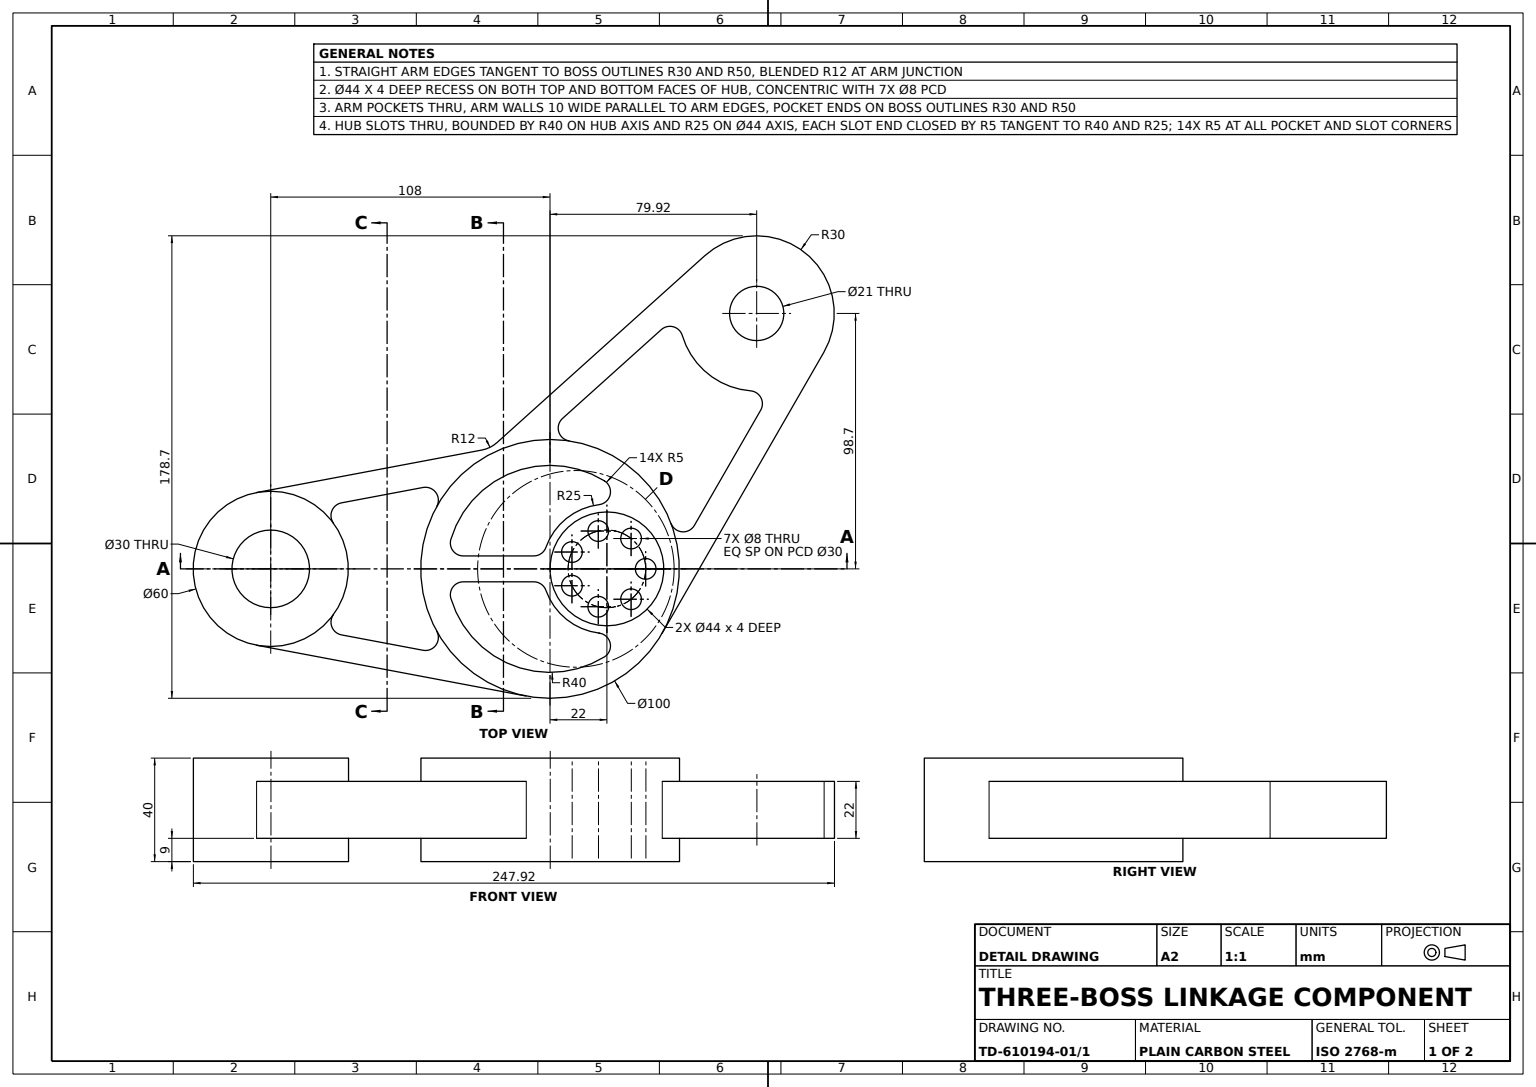
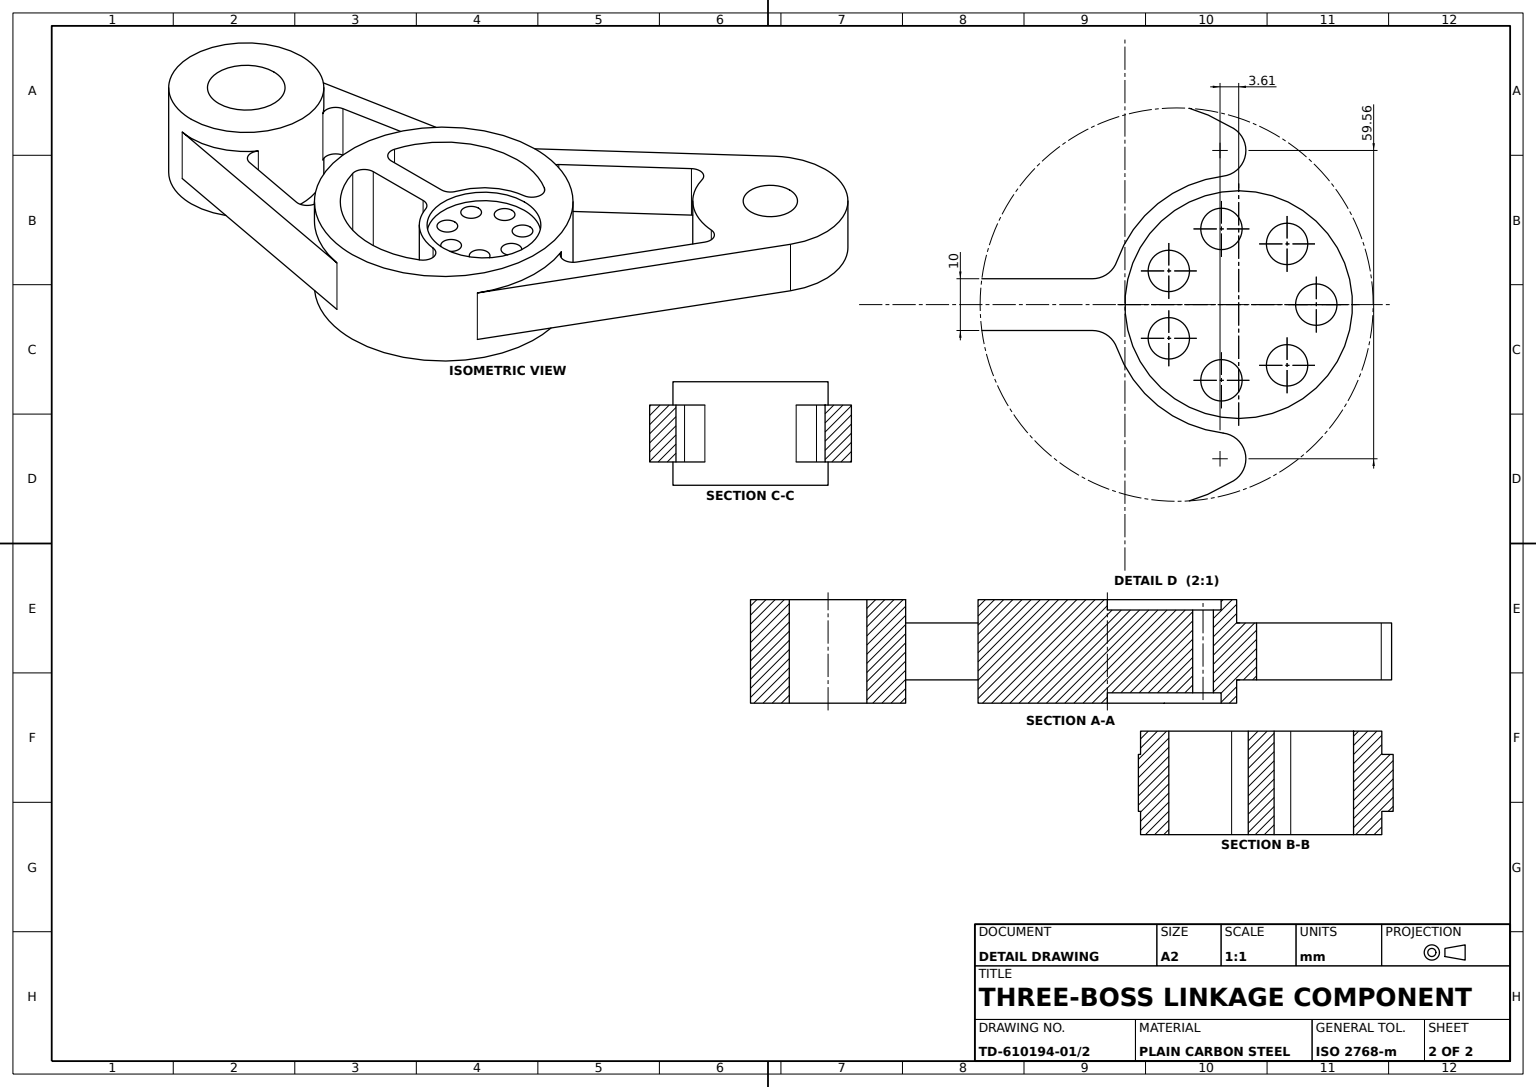
from build123d import *

# Parameters (mm, degrees)
HUB_AND_ARM_PROFILE_SKETCH_R   = 50
HUB_AND_ARM_PROFILE_SKETCH_R_2 = 4
HUB_AND_ARM_BODY_DEPTH         = 20
HUB_AND_ARM_PROFILE_SKETCH_R_3 = 30
HUB_AND_ARM_PROFILE_SKETCH_R_4 = 15
HUB_AND_ARM_BODY_2_DEPTH       = 20
HUB_RECESS_SKETCH_R            = 22
HUB_RECESS_DEPTH               = 4
ANGLED_ARM_SKETCH_R            = 30
ANGLED_ARM_SKETCH_R_2          = 10.5
ANGLED_ARM_BOSS_DEPTH          = 11
ARM_WALL_SKETCH_1_R            = 15
ARM_WALL_SKETCH_1_R_2          = 22
ARM_WALL_BOSS_1_DEPTH          = 11
ARM_WALL_SKETCH_2_R            = 10.5
ARM_WALL_SKETCH_2_R_2          = 22
ARM_WALL_BOSS_2_DEPTH          = 11


with BuildPart() as part:
    # Hub and Arm Profile Sketch → Hub and Arm Body (new, symmetric)
    with BuildSketch(Plane(origin=(0, 0, 0), x_dir=(1, 0, 0), z_dir=(0, 1, 0))):
        with Locations(Location((0, 0, 0), (0, 0, 270))):
            Circle(HUB_AND_ARM_PROFILE_SKETCH_R)
        with Locations(Location((37, 0, 0), (0, 0, 270))):
            Circle(HUB_AND_ARM_PROFILE_SKETCH_R_2, mode=Mode.SUBTRACT)
        with Locations(Location((31.352347028, -11.727472237, 0), (0, 0, 270))):
            Circle(HUB_AND_ARM_PROFILE_SKETCH_R_2, mode=Mode.SUBTRACT)
        with Locations(Location((18.662185991, -14.623918683, 0), (0, 0, 270))):
            Circle(HUB_AND_ARM_PROFILE_SKETCH_R_2, mode=Mode.SUBTRACT)
        with Locations(Location((8.485466981, -6.508256087, 0), (0, 0, 270))):
            Circle(HUB_AND_ARM_PROFILE_SKETCH_R_2, mode=Mode.SUBTRACT)
        with Locations(Location((8.485466981, 6.508256087, 0), (0, 0, 270))):
            Circle(HUB_AND_ARM_PROFILE_SKETCH_R_2, mode=Mode.SUBTRACT)
        with Locations(Location((18.662185991, 14.623918683, 0), (0, 0, 270))):
            Circle(HUB_AND_ARM_PROFILE_SKETCH_R_2, mode=Mode.SUBTRACT)
        with Locations(Location((31.352347028, 11.727472237, 0), (0, 0, 270))):
            Circle(HUB_AND_ARM_PROFILE_SKETCH_R_2, mode=Mode.SUBTRACT)
        with BuildLine():
            Line((-33.541019662, 5), (-6.284271247, 5))
            ThreePointArc((-6.284271247, 5), (-3.397519902, 5.917517095), (-1.57022604, 8.333333333))
            ThreePointArc((-1.57022604, 8.333333333), (6.360912817, 19.504331623), (18.988636364, 24.817971091))
            ThreePointArc((18.988636364, 24.817971091), (23.269989417, 28.70909189), (21.012987013, 34.036074638))
            ThreePointArc((21.012987013, 34.036074638), (-14.239627665, 37.37958004), (-38.3325939, 11.428571429))
            ThreePointArc((-38.3325939, 11.428571429), (-37.549938291, 7.011928477), (-33.541019662, 5))
        make_face(mode=Mode.SUBTRACT)
        with BuildLine():
            Line((-33.541019662, -5), (-6.284271247, -5))
            ThreePointArc((-6.284271247, -5), (-3.397519902, -5.917517095), (-1.57022604, -8.333333333))
            ThreePointArc((-1.57022604, -8.333333333), (6.360912817, -19.504331623), (18.988636364, -24.817971091))
            ThreePointArc((18.988636364, -24.817971091), (23.269989417, -28.70909189), (21.012987013, -34.036074638))
            ThreePointArc((21.012987013, -34.036074638), (-14.239627665, -37.37958004), (-38.3325939, -11.428571429))
            ThreePointArc((-38.3325939, -11.428571429), (-37.549938291, -7.011928477), (-33.541019662, -5))
        make_face(mode=Mode.SUBTRACT)
    extrude(amount=HUB_AND_ARM_BODY_DEPTH, both=True)

    # Hub Recess Sketch → Hub Recess (cut)
    with BuildSketch(Plane(origin=(0, 20, 0), x_dir=(1, 0, 0), z_dir=(0, 1, 0))):
        with Locations(Location((22, 0, 0), (0, 0, 270))):
            Circle(HUB_RECESS_SKETCH_R)
    hub_recess = extrude(amount=-HUB_RECESS_DEPTH, mode=Mode.SUBTRACT)

    # Hub Recess Mirror: Hub Recess across plane
    add(hub_recess.mirror(Plane.ZX), mode=Mode.SUBTRACT)



with BuildPart() as body_2:
    # Hub and Arm Profile Sketch → Hub and Arm Body 2 (new, symmetric)
    with BuildSketch(Plane(origin=(0, 0, 0), x_dir=(1, 0, 0), z_dir=(0, 1, 0))):
        with Locations(Location((-108, 0, 0), (0, 0, 270))):
            Circle(HUB_AND_ARM_PROFILE_SKETCH_R_3)
        with Locations(Location((-108, 0, 0), (0, 0, 270))):
            Circle(HUB_AND_ARM_PROFILE_SKETCH_R_4, mode=Mode.SUBTRACT)
    extrude(amount=HUB_AND_ARM_BODY_2_DEPTH, both=True)


with BuildPart() as body_3:
    # Angled Arm Sketch → Angled Arm Boss (new, symmetric)
    with BuildSketch(Plane(origin=(0, 0, 0), x_dir=(1, 0, 0), z_dir=(0, 1, 0))):
        with Locations(Location((79.923689663, 98.697537105, 0), (0, 0, 270))):
            Circle(ANGLED_ARM_SKETCH_R)
        with Locations(Location((79.923689663, 98.697537105, 0), (0, 0, 270))):
            Circle(ANGLED_ARM_SKETCH_R_2, mode=Mode.SUBTRACT)
    extrude(amount=ANGLED_ARM_BOSS_DEPTH, both=True)


with BuildPart() as part_1:
    add(part.part)

    add(body_2.part)  # Arm Wall Boss 1 merges body 2
    # Arm Wall Sketch 1 → Arm Wall Boss 1 (add, symmetric)
    with BuildSketch(Plane(origin=(0, 0, 0), x_dir=(1, 0, 0), z_dir=(0, 1, 0))):
        with BuildLine():
            Line((-113.555555556, -29.481109248), (-9.259259259, -49.135182079))
            ThreePointArc((-9.259259259, -49.135182079), (50, 0), (-9.259259259, 49.135182079))
            Line((-9.259259259, 49.135182079), (-113.555555556, 29.481109248))
            ThreePointArc((-113.555555556, 29.481109248), (-138, 0), (-113.555555556, -29.481109248))
        make_face()
        with Locations(Location((-108, 0, 0), (0, 0, 270))):
            Circle(ARM_WALL_SKETCH_1_R, mode=Mode.SUBTRACT)
        with Locations(Location((22, 0, 0), (0, 0, 270))):
            Circle(ARM_WALL_SKETCH_1_R_2, mode=Mode.SUBTRACT)
        with BuildLine():
            Line((-80.62788598, -25.510142573), (-49.099991939, -31.45140365))
            ThreePointArc((-49.099991939, -31.45140365), (-44.12443771, -29.470548159), (-43.794605467, -24.125350402))
            ThreePointArc((-43.794605467, -24.125350402), (-50, 0), (-43.794605467, 24.125350402))
            ThreePointArc((-43.794605467, 24.125350402), (-44.12443771, 29.470548159), (-49.099991939, 31.45140365))
            Line((-49.099991939, 31.45140365), (-80.62788598, 25.510142573))
            ThreePointArc((-80.62788598, 25.510142573), (-84.349569099, 22.440460086), (-83.744537189, 17.654249456))
            ThreePointArc((-83.744537189, 17.654249456), (-78, 0), (-83.744537189, -17.654249456))
            ThreePointArc((-83.744537189, -17.654249456), (-84.349569099, -22.440460086), (-80.62788598, -25.510142573))
        make_face(mode=Mode.SUBTRACT)
        with BuildLine():
            Line((-6.284271247, -5), (-33.541019662, -5))
            ThreePointArc((-33.541019662, -5), (-37.549938291, -7.011928477), (-38.3325939, -11.428571429))
            ThreePointArc((-38.3325939, -11.428571429), (-14.239627665, -37.37958004), (21.012987013, -34.036074638))
            ThreePointArc((21.012987013, -34.036074638), (23.269989417, -28.70909189), (18.988636364, -24.817971091))
            ThreePointArc((18.988636364, -24.817971091), (6.360912817, -19.504331623), (-1.57022604, -8.333333333))
            ThreePointArc((-1.57022604, -8.333333333), (-3.397519902, -5.917517095), (-6.284271247, -5))
        make_face(mode=Mode.SUBTRACT)
        with BuildLine():
            Line((-33.541019662, 5), (-6.284271247, 5))
            ThreePointArc((-6.284271247, 5), (-3.397519902, 5.917517095), (-1.57022604, 8.333333333))
            ThreePointArc((-1.57022604, 8.333333333), (6.360912817, 19.504331623), (18.988636364, 24.817971091))
            ThreePointArc((18.988636364, 24.817971091), (23.269989417, 28.70909189), (21.012987013, 34.036074638))
            ThreePointArc((21.012987013, 34.036074638), (-14.239627665, 37.37958004), (-38.3325939, 11.428571429))
            ThreePointArc((-38.3325939, 11.428571429), (-37.549938291, 7.011928477), (-33.541019662, 5))
        make_face(mode=Mode.SUBTRACT)
    extrude(amount=ARM_WALL_BOSS_1_DEPTH, both=True)


    add(body_3.part)  # Arm Wall Boss 2 merges body 3
    # Arm Wall Sketch 2 → Arm Wall Boss 2 (add, symmetric)
    with BuildSketch(Plane(origin=(0, 0, 0), x_dir=(1, 0, 0), z_dir=(0, 1, 0))):
        with BuildLine():
            Line((-49.099991939, 31.45140365), (-80.62788598, 25.510142573))
            ThreePointArc((-80.62788598, 25.510142573), (-84.349569099, 22.440460086), (-83.744537189, 17.654249456))
            ThreePointArc((-83.744537189, 17.654249456), (-96.936985674, 27.885654269), (-113.555555556, 29.481109248))
            Line((-113.555555556, 29.481109248), (-26.309191814, 45.922214523))
            ThreePointArc((-26.309191814, 45.922214523), (-23.213503206, 46.957343297), (-20.511294927, 48.788422203))
            Line((-20.511294927, 48.788422203), (59.873391891, 121.013127154))
            ThreePointArc((59.873391891, 121.013127154), (98.803301395, 122.011915949), (105.92032184, 83.725058503))
            Line((105.92032184, 83.725058503), (43.327720294, -24.954131003))
            ThreePointArc((43.327720294, -24.954131003), (-24.540851028, -43.56313385), (-43.794605467, 24.125350402))
            ThreePointArc((-43.794605467, 24.125350402), (-44.12443771, 29.470548159), (-49.099991939, 31.45140365))
        make_face()
        with Locations(Location((79.923689663, 98.697537105, 0), (0, 0, 270))):
            Circle(ARM_WALL_SKETCH_2_R, mode=Mode.SUBTRACT)
        with Locations(Location((22, 0, 0), (0, 0, 270))):
            Circle(ARM_WALL_SKETCH_2_R_2, mode=Mode.SUBTRACT)
        with BuildLine():
            Line((55.836458536, 16.801484997), (81.472399581, 61.313028313))
            ThreePointArc((81.472399581, 61.313028313), (81.564600618, 66.136447721), (77.53735071, 68.792597941))
            ThreePointArc((77.53735071, 68.792597941), (61.044077932, 75.383158261), (51.168392937, 90.145758918))
            ThreePointArc((51.168392937, 90.145758918), (47.732973634, 93.532759069), (43.034127187, 92.439727562))
            Line((43.034127187, 92.439727562), (4.825279735, 58.109523105))
            ThreePointArc((4.825279735, 58.109523105), (3.377881635, 52.953461905), (7.424541846, 49.445689179))
            ThreePointArc((7.424541846, 49.445689179), (31.466019552, 38.857298073), (46.821533188, 17.542634634))
            ThreePointArc((46.821533188, 17.542634634), (51.09400063, 14.313710616), (55.836458536, 16.801484997))
        make_face(mode=Mode.SUBTRACT)
        with BuildLine():
            Line((-33.541019662, 5), (-6.284271247, 5))
            ThreePointArc((-6.284271247, 5), (-3.397519902, 5.917517095), (-1.57022604, 8.333333333))
            ThreePointArc((-1.57022604, 8.333333333), (6.360912817, 19.504331623), (18.988636364, 24.817971091))
            ThreePointArc((18.988636364, 24.817971091), (23.269989417, 28.70909189), (21.012987013, 34.036074638))
            ThreePointArc((21.012987013, 34.036074638), (-14.239627665, 37.37958004), (-38.3325939, 11.428571429))
            ThreePointArc((-38.3325939, 11.428571429), (-37.549938291, 7.011928477), (-33.541019662, 5))
        make_face(mode=Mode.SUBTRACT)
        with BuildLine():
            Line((-6.284271247, -5), (-33.541019662, -5))
            ThreePointArc((-33.541019662, -5), (-37.549938291, -7.011928477), (-38.3325939, -11.428571429))
            ThreePointArc((-38.3325939, -11.428571429), (-14.239627665, -37.37958004), (21.012987013, -34.036074638))
            ThreePointArc((21.012987013, -34.036074638), (23.269989417, -28.70909189), (18.988636364, -24.817971091))
            ThreePointArc((18.988636364, -24.817971091), (6.360912817, -19.504331623), (-1.57022604, -8.333333333))
            ThreePointArc((-1.57022604, -8.333333333), (-3.397519902, -5.917517095), (-6.284271247, -5))
        make_face(mode=Mode.SUBTRACT)
    extrude(amount=ARM_WALL_BOSS_2_DEPTH, both=True)


solid = part_1.part
